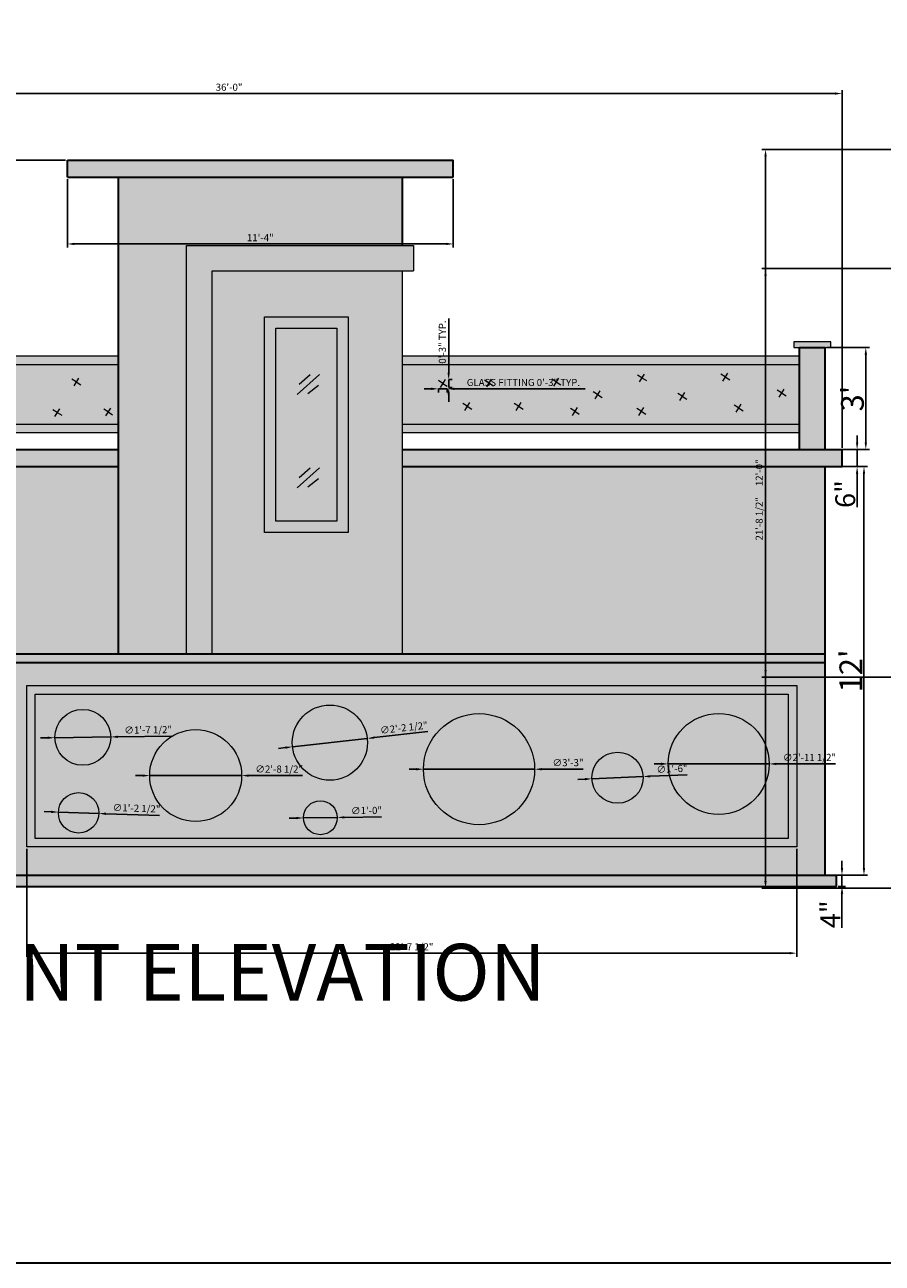
# Model space of a CAD drawing. Units: inches. Extents: x 2163 to 7246, y 928 to 2098.
# Tile 2 of 15: x 2404 to 2706, y 928 to 1365. Entities that reach past the tile are written whole.
import ezdxf

# ---------------------------------------------------------------- set-up
doc = ezdxf.new("R2010")
doc.units = ezdxf.units.IN
for name, color, linetype, lineweight in [('A-ANNO-DIMS', 4, 'Continuous', 18), ('A-ANNO-TITL', 4, 'Continuous', 30), ('A-ANNO-TTLB', 7, 'Continuous', 30), ('A-ELEV', 7, 'Continuous', 30), ('A-ELEV-DETL', 7, 'Continuous', 18), ('A-GLAZ', 30, 'Continuous', 20)]:
    doc.layers.add(name, color=color, linetype=linetype, lineweight=lineweight)
for name, color, linetype, lineweight, true_color in [('A-ELEV-PATT', 254, 'Continuous', 9, 0xd7ebd2), ('A-ELEV-TRIM-PATT', 11, 'Continuous', 9, 0xf27172), ('A-GLAZ-PATT', 141, 'Continuous', 9, 0xadddf7)]:
    doc.layers.add(name, color=color, linetype=linetype, lineweight=lineweight, true_color=true_color)
doc.styles.get("Standard").update_dxf_attribs({"font": 'arial.ttf'})
doc.dimstyles.new('ISO-25', dxfattribs={"dimtxt": 2.5, "dimasz": 2.5, "dimexe": 1.25, "dimexo": 0.625, "dimtad": 1, "dimdec": 0, "dimlunit": 3, "dimtxsty": 'Standard', "dimcen": 2.5, "dimadec": 0, "dimazin": 0, "dimtfac": 1, "dimtdec": 0, "dimtmove": 0, "dimatfit": 3, "dimfxl": 1, "dimarcsym": 0})

# ---------------------------------------------------------------- blocks, each defined once
blk = doc.blocks.new('*D21')
at = {"layer": 'A-ANNO-DIMS', "color": 0, "lineweight": -2, "transparency": 16777216}
for p, q in [((2691.82, 1067.77), (2691.82, 1070.27)), ((2690.47, 1065.27), (2693.07, 1065.27)), ((2691.82, 1065.27), (2691.82, 1061.27)), ((2690.47, 1061.27), (2693.07, 1061.27)), ((2691.82, 1058.77), (2691.82, 1046.7))]:
    blk.add_line(p, q, dxfattribs=at)
at = {"layer": 'A-ANNO-DIMS', "color": 0, "transparency": 16777216}
for points in [[(2691.4, 1067.77), (2692.24, 1067.77), (2691.82, 1065.27)], [(2691.4, 1058.77), (2692.24, 1058.77), (2691.82, 1061.27)]]:
    blk.add_solid(points, dxfattribs=at)
at = {"layer": 'Defpoints', "color": 0, "transparency": 16777216}
for p in [(2689.84, 1065.27), (2689.84, 1061.27), (2691.82, 1061.27)]:
    blk.add_point(p, dxfattribs=at)
at = {"layer": 'A-ANNO-DIMS', "color": 0, "transparency": 16777216, "insert": (2687.7, 1051.48), "char_height": 2.5, "attachment_point": 5, "rotation": 90}
blk.add_mtext('{\\H2.8x;4"}', dxfattribs=at)
blk = doc.blocks.new('*D22')
at = {"layer": 'A-ANNO-DIMS', "color": 0, "lineweight": -2, "transparency": 16777216}
for p, q in [((2686.47, 1209.27), (2700.82, 1209.27)), ((2699.57, 1206.77), (2699.57, 1067.77)), ((2686.47, 1065.27), (2700.82, 1065.27))]:
    blk.add_line(p, q, dxfattribs=at)
at = {"layer": 'A-ANNO-DIMS', "color": 0, "transparency": 16777216}
for points in [[(2699.15, 1206.77), (2699.98, 1206.77), (2699.57, 1209.27)], [(2699.15, 1067.77), (2699.98, 1067.77), (2699.57, 1065.27)]]:
    blk.add_solid(points, dxfattribs=at)
at = {"layer": 'Defpoints', "color": 0, "transparency": 16777216}
for p in [(2685.84, 1209.27), (2685.84, 1065.27), (2699.57, 1065.27)]:
    blk.add_point(p, dxfattribs=at)
at = {"layer": 'A-ANNO-DIMS', "color": 0, "transparency": 16777216, "insert": (2694.93, 1137.27), "char_height": 2.5, "attachment_point": 5, "rotation": 90}
blk.add_mtext("{\\H3.2x;12'}", dxfattribs=at)
blk = doc.blocks.new('*D23')
at = {"layer": 'A-ANNO-DIMS', "color": 0, "lineweight": -2, "transparency": 16777216}
for p, q in [((2697.15, 1217.77), (2697.15, 1220.27)), ((2692.47, 1215.27), (2698.4, 1215.27)), ((2697.15, 1215.27), (2697.15, 1209.27)), ((2692.47, 1209.27), (2698.4, 1209.27)), ((2697.15, 1206.77), (2697.15, 1194.94))]:
    blk.add_line(p, q, dxfattribs=at)
at = {"layer": 'A-ANNO-DIMS', "color": 0, "transparency": 16777216}
for points in [[(2696.74, 1217.77), (2697.57, 1217.77), (2697.15, 1215.27)], [(2696.74, 1206.77), (2697.57, 1206.77), (2697.15, 1209.27)]]:
    blk.add_solid(points, dxfattribs=at)
at = {"layer": 'Defpoints', "color": 0, "transparency": 16777216}
for p in [(2691.84, 1215.27), (2691.84, 1209.27), (2697.15, 1209.27)]:
    blk.add_point(p, dxfattribs=at)
at = {"layer": 'A-ANNO-DIMS', "color": 0, "transparency": 16777216, "insert": (2692.96, 1199.61), "char_height": 2.5, "attachment_point": 5, "rotation": 90}
blk.add_mtext('{\\H2.8x;6"}', dxfattribs=at)
blk = doc.blocks.new('*D24')
at = {"layer": 'A-ANNO-DIMS', "color": 0, "lineweight": -2, "transparency": 16777216}
for p, q in [((2686.47, 1251.27), (2701.46, 1251.27)), ((2700.21, 1248.77), (2700.21, 1217.77)), ((2686.47, 1215.27), (2701.46, 1215.27))]:
    blk.add_line(p, q, dxfattribs=at)
at = {"layer": 'A-ANNO-DIMS', "color": 0, "transparency": 16777216}
for points in [[(2699.8, 1248.77), (2700.63, 1248.77), (2700.21, 1251.27)], [(2699.8, 1217.77), (2700.63, 1217.77), (2700.21, 1215.27)]]:
    blk.add_solid(points, dxfattribs=at)
at = {"layer": 'Defpoints', "color": 0, "transparency": 16777216}
for p in [(2685.84, 1251.27), (2685.84, 1215.27), (2700.21, 1215.27)]:
    blk.add_point(p, dxfattribs=at)
at = {"layer": 'A-ANNO-DIMS', "color": 0, "transparency": 16777216, "insert": (2695.5, 1233.27), "char_height": 2.5, "attachment_point": 5, "rotation": 90}
blk.add_mtext("{\\H3.2x;3'}", dxfattribs=at)
blk = doc.blocks.new('GLASS-PANEL-FITTING')
for p, q in [((1.52, 1.46), (0, 2.43)), ((2.35, 2.77), (0.6, 0)), ((1.52, 1.46), (3.15, 0.44))]:
    blk.add_line(p, q)
blk = doc.blocks.new('GLAZ-REFLECTION')
for p, q in [((0, 0), (7.81, 7.08)), ((0.72, 3.7), (4.52, 7.08)), ((3.8, 0.41), (7.5, 3.29))]:
    blk.add_line(p, q)
blk = doc.blocks.new('*D47')
at = {"layer": 'A-ANNO-DIMS', "color": 0, "lineweight": -2, "transparency": 16777216}
for p, q in [((2547.09, 1236.69), (2544.59, 1236.69)), ((2549.59, 1236.69), (2552.74, 1236.69)), ((2549.59, 1236.54), (2549.59, 1235.44)), ((2552.74, 1236.54), (2552.74, 1235.44)), ((2555.24, 1236.69), (2601.36, 1236.69))]:
    blk.add_line(p, q, dxfattribs=at)
at = {"layer": 'A-ANNO-DIMS', "color": 0, "transparency": 16777216}
for points in [[(2547.09, 1237.11), (2547.09, 1236.28), (2549.59, 1236.69)], [(2555.24, 1237.11), (2555.24, 1236.28), (2552.74, 1236.69)]]:
    blk.add_solid(points, dxfattribs=at)
at = {"layer": 'Defpoints', "color": 0, "transparency": 16777216}
for p in [(2549.59, 1237.17), (2552.74, 1237.17), (2552.74, 1236.69)]:
    blk.add_point(p, dxfattribs=at)
at = {"layer": 'A-ANNO-DIMS', "color": 0, "transparency": 16777216, "insert": (2579.55, 1238.61), "char_height": 2.5, "attachment_point": 5}
blk.add_mtext('GLASS FITTING 0\'-3" TYP.', dxfattribs=at)
blk = doc.blocks.new('*D48')
at = {"layer": 'A-ANNO-DIMS', "color": 0, "lineweight": -2, "transparency": 16777216}
for p, q in [((2553.22, 1242.44), (2553.22, 1261.43)), ((2553.22, 1237.17), (2553.22, 1239.94)), ((2553.37, 1239.94), (2554.47, 1239.94)), ((2553.37, 1237.17), (2554.47, 1237.17)), ((2553.22, 1234.67), (2553.22, 1232.17))]:
    blk.add_line(p, q, dxfattribs=at)
at = {"layer": 'A-ANNO-DIMS', "color": 0, "transparency": 16777216}
for points in [[(2552.8, 1242.44), (2553.63, 1242.44), (2553.22, 1239.94)], [(2552.8, 1234.67), (2553.63, 1234.67), (2553.22, 1237.17)]]:
    blk.add_solid(points, dxfattribs=at)
at = {"layer": 'Defpoints', "color": 0, "transparency": 16777216}
for p in [(2552.74, 1239.94), (2553.22, 1239.94), (2552.74, 1237.17)]:
    blk.add_point(p, dxfattribs=at)
at = {"layer": 'A-ANNO-DIMS', "color": 0, "transparency": 16777216, "insert": (2551.31, 1253.18), "char_height": 2.5, "attachment_point": 5, "rotation": 90}
blk.add_mtext('0\'-3" TYP.', dxfattribs=at)
blk = doc.blocks.new('*D93')
at = {"layer": 'A-ANNO-DIMS', "color": 0, "lineweight": -2, "transparency": 16777216}
for p, q in [((2259.84, 1215.9), (2259.84, 1342.02)), ((2262.34, 1340.77), (2689.34, 1340.77)), ((2691.84, 1215.9), (2691.84, 1342.02))]:
    blk.add_line(p, q, dxfattribs=at)
at = {"layer": 'A-ANNO-DIMS', "color": 0, "transparency": 16777216}
for points in [[(2262.34, 1341.19), (2262.34, 1340.36), (2259.84, 1340.77)], [(2689.34, 1341.19), (2689.34, 1340.36), (2691.84, 1340.77)]]:
    blk.add_solid(points, dxfattribs=at)
at = {"layer": 'Defpoints', "color": 0, "transparency": 16777216}
for p in [(2691.84, 1340.77), (2259.84, 1215.27), (2691.84, 1215.27)]:
    blk.add_point(p, dxfattribs=at)
at = {"layer": 'A-ANNO-DIMS', "color": 0, "transparency": 16777216, "insert": (2475.84, 1342.68), "char_height": 2.5, "attachment_point": 5}
blk.add_mtext('36\'-0"', dxfattribs=at)
blk = doc.blocks.new('*D94')
at = {"layer": 'A-ANNO-DIMS', "color": 0, "lineweight": -2, "transparency": 16777216}
for p, q in [((2418.22, 1317.27), (2235.09, 1317.27)), ((2236.34, 1314.77), (2236.34, 1063.77)), ((2261.22, 1061.27), (2235.09, 1061.27))]:
    blk.add_line(p, q, dxfattribs=at)
at = {"layer": 'A-ANNO-DIMS', "color": 0, "transparency": 16777216}
for points in [[(2235.93, 1314.77), (2236.76, 1314.77), (2236.34, 1317.27)], [(2235.93, 1063.77), (2236.76, 1063.77), (2236.34, 1061.27)]]:
    blk.add_solid(points, dxfattribs=at)
at = {"layer": 'Defpoints', "color": 0, "transparency": 16777216}
for p in [(2418.84, 1317.27), (2236.34, 1061.27), (2261.84, 1061.27)]:
    blk.add_point(p, dxfattribs=at)
at = {"layer": 'A-ANNO-DIMS', "color": 0, "transparency": 16777216, "insert": (2234.46, 1189.27), "char_height": 2.5, "attachment_point": 5, "rotation": 90}
blk.add_mtext('21\'-4"', dxfattribs=at)
blk = doc.blocks.new('*D95')
at = {"layer": 'A-ANNO-DIMS', "color": 0, "lineweight": -2, "transparency": 16777216}
for p, q in [((2418.84, 1310.65), (2418.84, 1286.52)), ((2554.84, 1310.65), (2554.84, 1286.52)), ((2552.34, 1287.77), (2421.34, 1287.77))]:
    blk.add_line(p, q, dxfattribs=at)
at = {"layer": 'A-ANNO-DIMS', "color": 0, "transparency": 16777216}
for points in [[(2421.34, 1288.19), (2421.34, 1287.36), (2418.84, 1287.77)], [(2552.34, 1288.19), (2552.34, 1287.36), (2554.84, 1287.77)]]:
    blk.add_solid(points, dxfattribs=at)
at = {"layer": 'Defpoints', "color": 0, "transparency": 16777216}
for p in [(2418.84, 1311.27), (2554.84, 1311.27), (2418.84, 1287.77)]:
    blk.add_point(p, dxfattribs=at)
at = {"layer": 'A-ANNO-DIMS', "color": 0, "transparency": 16777216, "insert": (2486.84, 1289.65), "char_height": 2.5, "attachment_point": 5}
blk.add_mtext('11\'-4"', dxfattribs=at)
blk = doc.blocks.new('*D99')
at = {"layer": 'A-ANNO-DIMS', "color": 0, "lineweight": -2, "transparency": 16777216}
for p, q in [((2404.51, 1074.6), (2404.51, 1036.52)), ((2675.86, 1074.6), (2675.86, 1036.52)), ((2407.01, 1037.77), (2673.36, 1037.77))]:
    blk.add_line(p, q, dxfattribs=at)
at = {"layer": 'A-ANNO-DIMS', "color": 0, "transparency": 16777216}
for points in [[(2407.01, 1038.19), (2407.01, 1037.36), (2404.51, 1037.77)], [(2673.36, 1038.19), (2673.36, 1037.36), (2675.86, 1037.77)]]:
    blk.add_solid(points, dxfattribs=at)
at = {"layer": 'Defpoints', "color": 0, "transparency": 16777216}
for p in [(2404.51, 1075.23), (2675.86, 1075.23), (2675.86, 1037.77)]:
    blk.add_point(p, dxfattribs=at)
at = {"layer": 'A-ANNO-DIMS', "color": 0, "transparency": 16777216, "insert": (2540.19, 1039.69), "char_height": 2.5, "attachment_point": 5}
blk.add_mtext('22\'-7 1/2"', dxfattribs=at)
blk = doc.blocks.new('*D101')
at = {"layer": 'A-ANNO-DIMS', "color": 0, "lineweight": -2, "transparency": 16777216}
for p, q in [((2773.92, 1321.11), (2663.63, 1321.11)), ((2664.88, 1318.61), (2664.88, 1063.18)), ((2749.92, 1060.68), (2663.63, 1060.68))]:
    blk.add_line(p, q, dxfattribs=at)
at = {"layer": 'A-ANNO-DIMS', "color": 0, "transparency": 16777216}
for points in [[(2664.46, 1318.61), (2665.3, 1318.61), (2664.88, 1321.11)], [(2664.46, 1063.18), (2665.3, 1063.18), (2664.88, 1060.68)]]:
    blk.add_solid(points, dxfattribs=at)
at = {"layer": 'Defpoints', "color": 0, "transparency": 16777216}
for p in [(2774.54, 1321.11), (2664.88, 1060.68), (2750.54, 1060.68)]:
    blk.add_point(p, dxfattribs=at)
at = {"layer": 'A-ANNO-DIMS', "color": 0, "transparency": 16777216, "insert": (2662.96, 1190.89), "char_height": 2.5, "attachment_point": 5, "rotation": 90}
blk.add_mtext('21\'-8 1/2"', dxfattribs=at)
blk = doc.blocks.new('*D107')
at = {"layer": 'A-ANNO-DIMS', "color": 0, "lineweight": -2, "transparency": 16777216}
for p, q in [((3256.92, 1279.11), (2663.63, 1279.11)), ((2664.88, 1137.61), (2664.88, 1276.61)), ((3256.92, 1135.11), (2663.63, 1135.11))]:
    blk.add_line(p, q, dxfattribs=at)
at = {"layer": 'A-ANNO-DIMS', "color": 0, "transparency": 16777216}
for points in [[(2664.46, 1276.61), (2665.3, 1276.61), (2664.88, 1279.11)], [(2664.46, 1137.61), (2665.3, 1137.61), (2664.88, 1135.11)]]:
    blk.add_solid(points, dxfattribs=at)
at = {"layer": 'Defpoints', "color": 0, "transparency": 16777216}
for p in [(2664.88, 1279.11), (3257.54, 1279.11), (3257.54, 1135.11)]:
    blk.add_point(p, dxfattribs=at)
at = {"layer": 'A-ANNO-DIMS', "color": 0, "transparency": 16777216, "insert": (2662.98, 1207.11), "char_height": 2.5, "attachment_point": 5, "rotation": 90}
blk.add_mtext('12\'-0"', dxfattribs=at)
blk = doc.blocks.new('*D121')
at = {"layer": 'A-ANNO-DIMS', "color": 0, "lineweight": -2, "transparency": 16777216}
for p, q in [((2411.93, 1113.69), (2409.43, 1113.66)), ((2414.43, 1113.73), (2434.12, 1114)), ((2455.56, 1114.3), (2436.62, 1114.04))]:
    blk.add_line(p, q, dxfattribs=at)
at = {"layer": 'A-ANNO-DIMS', "color": 0, "transparency": 16777216}
for points in [[(2411.92, 1114.11), (2411.93, 1113.28), (2414.43, 1113.73)], [(2436.62, 1114.45), (2436.63, 1113.62), (2434.12, 1114)]]:
    blk.add_solid(points, dxfattribs=at)
at = {"layer": 'Defpoints', "color": 0, "transparency": 16777216}
for p in [(2414.43, 1113.73), (2434.12, 1114)]:
    blk.add_point(p, dxfattribs=at)
at = {"layer": 'A-ANNO-DIMS', "color": 0, "transparency": 16777216, "insert": (2447.32, 1116.16), "char_height": 2.5, "attachment_point": 5, "rotation": 0.7959}
blk.add_mtext('∅1\'-7 1/2"', dxfattribs=at)
blk = doc.blocks.new('*D122')
at = {"layer": 'A-ANNO-DIMS', "color": 0, "lineweight": -2, "transparency": 16777216}
for p, q in [((2413.19, 1087.57), (2410.69, 1087.66)), ((2415.68, 1087.49), (2429.93, 1087)), ((2451.36, 1086.27), (2432.43, 1086.92))]:
    blk.add_line(p, q, dxfattribs=at)
at = {"layer": 'A-ANNO-DIMS', "color": 0, "transparency": 16777216}
for points in [[(2413.2, 1087.99), (2413.17, 1087.15), (2415.68, 1087.49)], [(2432.45, 1087.33), (2432.42, 1086.5), (2429.93, 1087)]]:
    blk.add_solid(points, dxfattribs=at)
at = {"layer": 'Defpoints', "color": 0, "transparency": 16777216}
for p in [(2415.68, 1087.49), (2429.93, 1087)]:
    blk.add_point(p, dxfattribs=at)
at = {"layer": 'A-ANNO-DIMS', "color": 0, "transparency": 16777216, "insert": (2443.21, 1088.52), "char_height": 2.5, "attachment_point": 5, "rotation": 358.055}
blk.add_mtext('∅1\'-2 1/2"', dxfattribs=at)
blk = doc.blocks.new('*D123')
at = {"layer": 'A-ANNO-DIMS', "color": 0, "lineweight": -2, "transparency": 16777216}
for p, q in [((2445.37, 1100.37), (2442.87, 1100.37)), ((2447.87, 1100.37), (2480.27, 1100.37)), ((2501.71, 1100.37), (2482.77, 1100.37))]:
    blk.add_line(p, q, dxfattribs=at)
at = {"layer": 'A-ANNO-DIMS', "color": 0, "transparency": 16777216}
for points in [[(2445.37, 1100.78), (2445.37, 1099.95), (2447.87, 1100.37)], [(2482.77, 1100.78), (2482.77, 1099.95), (2480.27, 1100.37)]]:
    blk.add_solid(points, dxfattribs=at)
at = {"layer": 'Defpoints', "color": 0, "transparency": 16777216}
for p in [(2447.87, 1100.37), (2480.27, 1100.37)]:
    blk.add_point(p, dxfattribs=at)
at = {"layer": 'A-ANNO-DIMS', "color": 0, "transparency": 16777216, "insert": (2493.49, 1102.34), "char_height": 2.5, "attachment_point": 5, "rotation": 359.9996}
blk.add_mtext('∅2\'-8 1/2"', dxfattribs=at)
blk = doc.blocks.new('*D124')
at = {"layer": 'A-ANNO-DIMS', "color": 0, "lineweight": -2, "transparency": 16777216}
for p, q in [((2498.19, 1110.51), (2524.54, 1113.47)), ((2545.85, 1115.86), (2527.02, 1113.75)), ((2495.7, 1110.23), (2493.22, 1109.95))]:
    blk.add_line(p, q, dxfattribs=at)
at = {"layer": 'A-ANNO-DIMS', "color": 0, "transparency": 16777216}
for points in [[(2526.98, 1114.16), (2527.07, 1113.34), (2524.54, 1113.47)], [(2495.66, 1110.64), (2495.75, 1109.82), (2498.19, 1110.51)]]:
    blk.add_solid(points, dxfattribs=at)
at = {"layer": 'Defpoints', "color": 0, "transparency": 16777216}
for p in [(2524.54, 1113.47), (2498.19, 1110.51)]:
    blk.add_point(p, dxfattribs=at)
at = {"layer": 'A-ANNO-DIMS', "color": 0, "transparency": 16777216, "insert": (2537.46, 1116.91), "char_height": 2.5, "attachment_point": 5, "rotation": 6.4111}
blk.add_mtext('∅2\'-2 1/2"', dxfattribs=at)
blk = doc.blocks.new('*D125')
at = {"layer": 'A-ANNO-DIMS', "color": 0, "lineweight": -2, "transparency": 16777216}
for p, q in [((2499.52, 1085.4), (2497.02, 1085.37)), ((2502.02, 1085.44), (2513.98, 1085.61)), ((2529.59, 1085.83), (2516.48, 1085.64))]:
    blk.add_line(p, q, dxfattribs=at)
at = {"layer": 'A-ANNO-DIMS', "color": 0, "transparency": 16777216}
for points in [[(2499.51, 1085.82), (2499.52, 1084.99), (2502.02, 1085.44)], [(2516.47, 1086.06), (2516.49, 1085.23), (2513.98, 1085.61)]]:
    blk.add_solid(points, dxfattribs=at)
at = {"layer": 'Defpoints', "color": 0, "transparency": 16777216}
for p in [(2502.02, 1085.44), (2513.98, 1085.61)]:
    blk.add_point(p, dxfattribs=at)
at = {"layer": 'A-ANNO-DIMS', "color": 0, "transparency": 16777216, "insert": (2524.26, 1087.72), "char_height": 2.5, "attachment_point": 5, "rotation": 0.8105}
blk.add_mtext('∅1\'-0"', dxfattribs=at)
blk = doc.blocks.new('*D126')
at = {"layer": 'A-ANNO-DIMS', "color": 0, "lineweight": -2, "transparency": 16777216}
for p, q in [((2541.82, 1102.62), (2539.32, 1102.62)), ((2544.32, 1102.62), (2583.51, 1102.62)), ((2600.57, 1102.62), (2586.01, 1102.62))]:
    blk.add_line(p, q, dxfattribs=at)
at = {"layer": 'A-ANNO-DIMS', "color": 0, "transparency": 16777216}
for points in [[(2541.82, 1103.03), (2541.82, 1102.2), (2544.32, 1102.62)], [(2586.01, 1103.03), (2586.01, 1102.2), (2583.51, 1102.62)]]:
    blk.add_solid(points, dxfattribs=at)
at = {"layer": 'Defpoints', "color": 0, "transparency": 16777216}
for p in [(2544.32, 1102.62), (2583.51, 1102.62)]:
    blk.add_point(p, dxfattribs=at)
at = {"layer": 'A-ANNO-DIMS', "color": 0, "transparency": 16777216, "insert": (2595.27, 1104.59), "char_height": 2.5, "attachment_point": 5, "rotation": 0.0007}
blk.add_mtext('∅3\'-3"', dxfattribs=at)
blk = doc.blocks.new('*D127')
at = {"layer": 'A-ANNO-DIMS', "color": 0, "lineweight": -2, "transparency": 16777216}
for p, q in [((2637.31, 1100.69), (2624.21, 1100.12)), ((2601.22, 1099.12), (2598.72, 1099.01)), ((2603.72, 1099.23), (2621.71, 1100.01))]:
    blk.add_line(p, q, dxfattribs=at)
at = {"layer": 'A-ANNO-DIMS', "color": 0, "transparency": 16777216}
for points in [[(2624.19, 1100.53), (2624.23, 1099.7), (2621.71, 1100.01)], [(2601.2, 1099.53), (2601.24, 1098.7), (2603.72, 1099.23)]]:
    blk.add_solid(points, dxfattribs=at)
at = {"layer": 'Defpoints', "color": 0, "transparency": 16777216}
for p in [(2603.72, 1099.23), (2621.71, 1100.01)]:
    blk.add_point(p, dxfattribs=at)
at = {"layer": 'A-ANNO-DIMS', "color": 0, "transparency": 16777216, "insert": (2631.93, 1102.43), "char_height": 2.5, "attachment_point": 5, "rotation": 2.495}
blk.add_mtext('∅1\'-6"', dxfattribs=at)
blk = doc.blocks.new('*D128')
at = {"layer": 'A-ANNO-DIMS', "color": 0, "lineweight": -2, "transparency": 16777216}
for p, q in [((2628.09, 1104.49), (2625.59, 1104.49)), ((2630.59, 1104.49), (2666.17, 1104.49)), ((2689.55, 1104.49), (2668.67, 1104.49))]:
    blk.add_line(p, q, dxfattribs=at)
at = {"layer": 'A-ANNO-DIMS', "color": 0, "transparency": 16777216}
for points in [[(2628.09, 1104.91), (2628.09, 1104.08), (2630.59, 1104.49)], [(2668.67, 1104.91), (2668.67, 1104.07), (2666.17, 1104.49)]]:
    blk.add_solid(points, dxfattribs=at)
at = {"layer": 'Defpoints', "color": 0, "transparency": 16777216}
for p in [(2630.59, 1104.49), (2666.17, 1104.49)]:
    blk.add_point(p, dxfattribs=at)
at = {"layer": 'A-ANNO-DIMS', "color": 0, "transparency": 16777216, "insert": (2680.36, 1106.46), "char_height": 2.5, "attachment_point": 5, "rotation": 359.9986}
blk.add_mtext('∅2\'-11 1/2"', dxfattribs=at)

msp = doc.modelspace()

# ---------------------------------------------------------------- hatches: boundary and pattern name
at = {"layer": 'A-ELEV-PATT'}
h = msp.add_hatch(color=256, dxfattribs=at)
h.dxf.hatch_style = 1
h.paths.add_polyline_path([(2460.84, 1287.27), (2536.84, 1287.27), (2536.84, 1311.27), (2436.84, 1311.27), (2436.84, 1215.27), (2436.84, 1143.27), (2460.84, 1143.27), (2460.84, 1215.27)])
h = msp.add_hatch(color=256, dxfattribs=at)
h.dxf.hatch_style = 1
h.paths.add_polyline_path([(2536.84, 1278.27), (2469.84, 1278.27), (2469.84, 1215.27), (2469.84, 1143.27), (2536.84, 1143.27)])
h.paths.add_polyline_path([(2488.32, 1186.07), (2488.32, 1262.03), (2517.83, 1262.03), (2517.83, 1186.07)], flags=16)
h.paths.add_polyline_path([(2513.83, 1190.07), (2492.32, 1190.07), (2492.32, 1258.03), (2513.83, 1258.03)], flags=0)
h = msp.add_hatch(color=256, dxfattribs=at)
h.dxf.hatch_style = 1
h.paths.add_polyline_path([(2685.84, 1251.27), (2676.84, 1251.27), (2676.84, 1215.27), (2685.84, 1215.27)])
h = msp.add_hatch(color=256, dxfattribs=at)
h.dxf.hatch_style = 1
h.paths.add_polyline_path([(2436.84, 1209.27), (2265.84, 1209.27), (2265.84, 1143.27), (2319.84, 1143.27), (2319.84, 1140.27), (2313.84, 1140.27), (2313.84, 1125.27), (2355.84, 1125.27), (2355.84, 1137.27), (2385.84, 1137.27), (2385.84, 1140.27), (2379.84, 1140.27), (2379.84, 1143.27), (2436.84, 1143.27)])
h.paths.add_polyline_path([(2676.84, 1209.27), (2536.84, 1209.27), (2536.84, 1143.27), (2676.84, 1143.27)])
h = msp.add_hatch(color=256, dxfattribs=at)
h.dxf.hatch_style = 1
h.paths.add_polyline_path([(2685.84, 1209.27), (2536.84, 1209.27), (2536.84, 1143.27), (2676.84, 1143.27), (2685.84, 1143.27)])
h = msp.add_hatch(color=256, dxfattribs=at)
h.dxf.hatch_style = 1
h.paths.add_polyline_path([(2672.86, 1078.23), (2672.86, 1129.07), (2407.51, 1129.07), (2407.51, 1078.23)], flags=0)
h.paths.add_polyline_path([(2447.87, 1100.37, -1), (2480.27, 1100.37, -1)], flags=0)
h.paths.add_polyline_path([(2429.94, 1087.24, -1), (2415.68, 1087.24, -1)], flags=0)
h.paths.add_polyline_path([(2414.43, 1113.86, -1), (2434.12, 1113.86, -1)], flags=0)
h.paths.add_polyline_path([(2498.1, 1111.99, -1), (2524.62, 1111.99, -1)], flags=0)
h.paths.add_polyline_path([(2513.98, 1085.52, -1), (2502.02, 1085.52, -1)], flags=0)
h.paths.add_polyline_path([(2583.51, 1102.62, -1), (2544.32, 1102.62, -1)], flags=0)
h.paths.add_polyline_path([(2621.72, 1099.62, -1), (2603.71, 1099.62, -1)], flags=0)
h.paths.add_polyline_path([(2666.17, 1104.49, -1), (2630.59, 1104.49, -1)], flags=0)
h.paths.add_polyline_path([(2394.84, 1065.27), (2685.84, 1065.27), (2685.84, 1140.27), (2676.84, 1140.27), (2394.84, 1140.27)])
h.paths.add_polyline_path([(2404.51, 1132.07), (2675.86, 1132.07), (2675.86, 1075.23), (2404.51, 1075.23)], flags=16)
h.paths.add_polyline_path([(2407.51, 1129.07), (2672.86, 1129.07), (2672.86, 1078.23), (2407.51, 1078.23)], flags=0)
h = msp.add_hatch(color=256, dxfattribs=at)
h.dxf.hatch_style = 1
h.paths.add_polyline_path([(2672.86, 1078.23), (2672.86, 1129.07), (2407.51, 1129.07), (2407.51, 1078.23)])
h.paths.add_polyline_path([(2498.1, 1111.99, -1), (2524.62, 1111.99, -1)], flags=16)
h.paths.add_polyline_path([(2447.87, 1100.37, -1), (2480.27, 1100.37, -1)], flags=16)
h.paths.add_polyline_path([(2513.98, 1085.52, -1), (2502.02, 1085.52, -1)], flags=16)
h.paths.add_polyline_path([(2583.51, 1102.62, -1), (2544.32, 1102.62, -1)], flags=16)
h.paths.add_polyline_path([(2414.43, 1113.86, -1), (2434.12, 1113.86, -1)], flags=16)
h.paths.add_polyline_path([(2429.94, 1087.24, -1), (2415.68, 1087.24, -1)], flags=16)
h.paths.add_polyline_path([(2621.72, 1099.62, -1), (2603.71, 1099.62, -1)], flags=16)
h.paths.add_polyline_path([(2666.17, 1104.49, -1), (2630.59, 1104.49, -1)], flags=16)
at = {"layer": 'A-ELEV-TRIM-PATT'}
h = msp.add_hatch(color=256, dxfattribs=at)
h.dxf.hatch_style = 1
h.paths.add_polyline_path([(2418.84, 1317.27), (2418.84, 1311.27), (2554.84, 1311.27), (2554.84, 1317.27)])
h = msp.add_hatch(color=256, dxfattribs=at)
h.dxf.hatch_style = 1
h.paths.add_polyline_path([(2469.84, 1215.27), (2469.84, 1278.27), (2540.84, 1278.27), (2540.84, 1287.27), (2460.84, 1287.27), (2460.84, 1215.27), (2460.84, 1143.27), (2469.84, 1143.27)])
h = msp.add_hatch(color=256, dxfattribs=at)
h.dxf.hatch_style = 1
h.paths.add_polyline_path([(2488.32, 1186.07), (2517.83, 1186.07), (2517.83, 1262.03), (2488.32, 1262.03)])
h.paths.add_polyline_path([(2492.32, 1258.03), (2513.83, 1258.03), (2513.83, 1190.07), (2492.32, 1190.07)], flags=16)
h = msp.add_hatch(color=256, dxfattribs=at)
h.dxf.hatch_style = 1
h.paths.add_polyline_path([(2276.84, 1253.27), (2263.84, 1253.27), (2263.84, 1251.27), (2265.84, 1251.27), (2274.84, 1251.27), (2276.84, 1251.27)])
h.paths.add_polyline_path([(2687.84, 1253.27), (2676.84, 1253.27), (2674.84, 1253.27), (2674.84, 1251.27), (2676.84, 1251.27), (2685.84, 1251.27), (2687.84, 1251.27)])
h = msp.add_hatch(color=256, dxfattribs=at)
h.dxf.hatch_style = 1
h.paths.add_polyline_path([(2436.84, 1248.27), (2274.84, 1248.27), (2274.84, 1245.27), (2436.84, 1245.27)])
h.paths.add_polyline_path([(2436.84, 1224.27), (2274.84, 1224.27), (2274.84, 1221.27), (2436.84, 1221.27)])
h.paths.add_polyline_path([(2676.84, 1248.27), (2536.84, 1248.27), (2536.84, 1245.27), (2676.84, 1245.27)])
h.paths.add_polyline_path([(2676.84, 1224.27), (2536.84, 1224.27), (2536.84, 1221.27), (2676.84, 1221.27)])
h = msp.add_hatch(color=256, dxfattribs=at)
h.dxf.hatch_style = 1
h.paths.add_polyline_path([(2536.84, 1215.27), (2536.84, 1209.27), (2691.84, 1209.27), (2691.84, 1215.27)])
h.paths.add_polyline_path([(2259.84, 1215.27), (2259.84, 1209.27), (2436.84, 1209.27), (2436.84, 1215.27)])
h = msp.add_hatch(color=256, dxfattribs=at)
h.dxf.hatch_style = 1
h.paths.add_polyline_path([(2319.84, 1143.27), (2265.84, 1143.27), (2265.84, 1140.27), (2319.84, 1140.27)])
h.paths.add_polyline_path([(2676.84, 1143.27), (2379.84, 1143.27), (2379.84, 1140.27), (2676.84, 1140.27)])
h = msp.add_hatch(color=256, dxfattribs=at)
h.dxf.hatch_style = 1
h.paths.add_polyline_path([(2685.84, 1140.27), (2685.84, 1143.27), (2676.84, 1143.27), (2379.84, 1143.27), (2379.84, 1140.27), (2676.84, 1140.27)])
h = msp.add_hatch(color=256, dxfattribs=at)
h.dxf.hatch_style = 1
h.paths.add_polyline_path([(2404.51, 1075.23), (2675.86, 1075.23), (2675.86, 1132.07), (2404.51, 1132.07)])
h.paths.add_polyline_path([(2407.51, 1129.07), (2672.86, 1129.07), (2672.86, 1078.23), (2407.51, 1078.23)], flags=16)
h.paths.add_polyline_path([(2414.43, 1113.86, -1), (2434.12, 1113.86, -1)], flags=0)
h.paths.add_polyline_path([(2429.94, 1087.24, -1), (2415.68, 1087.24, -1)], flags=0)
h.paths.add_polyline_path([(2480.27, 1100.37, -1), (2447.87, 1100.37, -1)], flags=0)
h.paths.add_polyline_path([(2524.62, 1111.99, -1), (2498.1, 1111.99, -1)], flags=0)
h.paths.add_polyline_path([(2513.98, 1085.52, -1), (2502.02, 1085.52, -1)], flags=0)
h.paths.add_polyline_path([(2583.51, 1102.62, -1), (2544.32, 1102.62, -1)], flags=0)
h.paths.add_polyline_path([(2621.72, 1099.62, -1), (2603.71, 1099.62, -1)], flags=0)
h.paths.add_polyline_path([(2666.17, 1104.49, -1), (2630.59, 1104.49, -1)], flags=0)
h = msp.add_hatch(color=256, dxfattribs=at)
h.dxf.hatch_style = 1
h.paths.add_polyline_path([(2447.87, 1100.37, 1), (2480.27, 1100.37, 1)])
h.paths.add_polyline_path([(2524.62, 1111.99, 1), (2498.1, 1111.99, 1)])
h.paths.add_polyline_path([(2544.32, 1102.62, 1), (2583.51, 1102.62, 1)])
h.paths.add_polyline_path([(2603.71, 1099.62, 1), (2621.72, 1099.62, 1)])
h.paths.add_polyline_path([(2666.17, 1104.49, 1), (2630.59, 1104.49, 1)])
h.paths.add_polyline_path([(2415.68, 1087.24, 1), (2429.94, 1087.24, 1)])
h.paths.add_polyline_path([(2434.12, 1113.86, 1), (2414.43, 1113.86, 1)])
h = msp.add_hatch(color=256, dxfattribs=at)
h.dxf.hatch_style = 1
h.paths.add_polyline_path([(2502.02, 1085.52, 1), (2513.98, 1085.52, 1)])
h = msp.add_hatch(color=256, dxfattribs=at)
h.dxf.hatch_style = 1
h.paths.add_polyline_path([(2689.84, 1061.27), (2689.84, 1065.27), (2261.84, 1065.27), (2261.84, 1061.27)])
at = {"layer": 'A-GLAZ-PATT'}
h = msp.add_hatch(color=256, dxfattribs=at)
h.dxf.hatch_style = 1
h.paths.add_polyline_path([(2513.83, 1258.03), (2492.32, 1258.03), (2492.32, 1190.07), (2513.83, 1190.07)])
h = msp.add_hatch(color=256, dxfattribs=at)
h.dxf.hatch_style = 1
h.paths.add_polyline_path([(2436.84, 1224.27), (2436.84, 1245.27), (2274.84, 1245.27), (2274.84, 1224.27)])
h.paths.add_polyline_path([(2536.84, 1245.27), (2536.84, 1224.27), (2676.84, 1224.27), (2676.84, 1245.27)])

# ---------------------------------------------------------------- linework, layer by layer
at = {"layer": 'A-ANNO-TTLB'}
msp.add_lwpolyline([(2162.62, 2098.21), (3633.38, 2098.21), (3633.38, 928.48), (2162.62, 928.48)], close=True, dxfattribs=at)
at = {"layer": 'A-ELEV'}
for p, q in [((2418.84, 1317.27), (2554.84, 1317.27)), ((2418.84, 1311.27), (2418.84, 1317.27)), ((2554.84, 1311.27), (2554.84, 1317.27)), ((2418.84, 1311.27), (2554.84, 1311.27)), ((2436.84, 1215.27), (2436.84, 1311.27)), ((2536.84, 1311.27), (2536.84, 1287.27)), ((2676.84, 1251.27), (2685.84, 1251.27)), ((2676.84, 1215.27), (2676.84, 1251.27)), ((2685.84, 1215.27), (2685.84, 1251.27)), ((2259.84, 1215.27), (2436.84, 1215.27)), ((2436.84, 1143.27), (2436.84, 1215.27)), ((2536.84, 1215.27), (2691.84, 1215.27)), ((2691.84, 1209.27), (2691.84, 1215.27)), ((2259.84, 1209.27), (2436.84, 1209.27)), ((2536.84, 1209.27), (2691.84, 1209.27)), ((2685.84, 1065.27), (2685.84, 1209.27)), ((2379.84, 1143.27), (2676.84, 1143.27)), ((2379.84, 1140.27), (2676.84, 1140.27)), ((2676.84, 1143.27), (2685.84, 1143.27)), ((2676.84, 1140.27), (2685.84, 1140.27)), ((2261.84, 1065.27), (2689.84, 1065.27)), ((2689.84, 1061.27), (2689.84, 1065.27)), ((2261.84, 1061.27), (2689.84, 1061.27))]:
    msp.add_line(p, q, dxfattribs=at)
at = {"layer": 'A-ELEV-DETL'}
for p, q in [((2460.84, 1215.27), (2460.84, 1287.27)), ((2460.84, 1287.27), (2540.84, 1287.27)), ((2540.84, 1287.27), (2540.84, 1278.27)), ((2469.84, 1278.27), (2540.84, 1278.27)), ((2469.84, 1215.27), (2469.84, 1278.27)), ((2536.84, 1278.27), (2536.84, 1143.27)), ((2676.84, 1253.27), (2674.84, 1253.27)), ((2674.84, 1253.27), (2674.84, 1251.27)), ((2687.84, 1253.27), (2676.84, 1253.27)), ((2687.84, 1251.27), (2687.84, 1253.27)), ((2674.84, 1251.27), (2676.84, 1251.27)), ((2685.84, 1251.27), (2687.84, 1251.27)), ((2274.84, 1248.27), (2436.84, 1248.27)), ((2274.84, 1245.27), (2436.84, 1245.27)), ((2536.84, 1248.27), (2676.84, 1248.27)), ((2536.84, 1245.27), (2676.84, 1245.27)), ((2274.84, 1224.27), (2436.84, 1224.27)), ((2536.84, 1224.27), (2676.84, 1224.27)), ((2274.84, 1221.27), (2436.84, 1221.27)), ((2536.84, 1221.27), (2676.84, 1221.27)), ((2460.84, 1143.27), (2460.84, 1215.27)), ((2469.84, 1143.27), (2469.84, 1215.27))]:
    msp.add_line(p, q, dxfattribs=at)
for points in [[(2404.51, 1132.07), (2675.86, 1132.07), (2675.86, 1075.23), (2404.51, 1075.23)], [(2407.51, 1129.07), (2672.86, 1129.07), (2672.86, 1078.23), (2407.51, 1078.23)]]:
    msp.add_lwpolyline(points, close=True, dxfattribs=at)
for centre, radius in [((2424.28, 1113.86), 9.85), ((2511.36, 1111.99), 13.26), ((2563.92, 1102.62), 19.59), ((2648.38, 1104.49), 17.79), ((2464.07, 1100.37), 16.2), ((2612.72, 1099.62), 9.01), ((2422.81, 1087.24), 7.13), ((2508, 1085.52), 5.98)]:
    msp.add_circle(centre, radius, dxfattribs=at)
at = {"layer": 'A-GLAZ'}
for points in [[(2488.32, 1262.03), (2517.83, 1262.03), (2517.83, 1186.07), (2488.32, 1186.07)], [(2492.32, 1258.03), (2513.83, 1258.03), (2513.83, 1190.07), (2492.32, 1190.07)]]:
    msp.add_lwpolyline(points, close=True, dxfattribs=at)

# ---------------------------------------------------------------- block references
at = {"layer": 'A-ELEV-DETL'}
for p in [(2420.48, 1237.72), (2549.59, 1237.17), (2565.9, 1237.36), (2589.59, 1237.66), (2619.8, 1239.14), (2649.12, 1239.43), (2604.1, 1233.22), (2668.96, 1233.81), (2558.2, 1229.08), (2576.27, 1229.08), (2634.01, 1232.63), (2653.86, 1228.49), (2413.74, 1226.92), (2431.65, 1227.15), (2596.11, 1227.31), (2619.5, 1227.31)]:
    msp.add_blockref('GLASS-PANEL-FITTING', p, dxfattribs=at)
at = {"layer": 'A-GLAZ'}
for p in [(2499.84, 1234.64), (2499.84, 1201.79)]:
    msp.add_blockref('GLAZ-REFLECTION', p, dxfattribs=at)

# ---------------------------------------------------------------- texts
at = {"layer": 'A-ANNO-TITL', "insert": (2349.09, 1041.06), "char_height": 20, "attachment_point": 1}
msp.add_mtext_dynamic_manual_height_columns('FRONT ELEVATION', width=571.2399, gutter_width=12.5, heights=[0], dxfattribs=at)

# ---------------------------------------------------------------- dimensions: what is measured, and where the dimension line sits
at = {"layer": 'A-ANNO-DIMS'}
for base, p1, p2, picture, middle in [((2691.84, 1340.77), (2259.84, 1215.27), (2691.84, 1215.27), '*D93', (2475.84, 1342.68)), ((2675.8622, 1037.773), (2404.5127, 1075.2279), (2675.8622, 1075.2279), '*D99', (2540.1875, 1039.6907))]:
    dim = msp.add_linear_dim(base=base, p1=p1, p2=p2, dimstyle='ISO-25', override={"dimdec": 1, "dimlfac": 1, "dimrnd": 0, "dimzin": 1, "dimdsep": 46, "dimlunit": 4, "dimfrac": 2}, dxfattribs=at)
    dim.commit()
    dim.dimension.update_dxf_attribs({"geometry": picture, "text_midpoint": middle})
for base, p1, p2, angle, picture, middle in [((2664.88, 1060.68), (2774.54, 1321.11), (2750.54, 1060.68), 90, '*D101', (2662.96, 1190.89)), ((2236.34, 1061.27), (2418.84, 1317.27), (2261.84, 1061.27), 90, '*D94', (2234.46, 1189.27)), ((2418.84, 1287.77), (2554.84, 1311.27), (2418.84, 1311.27), 180, '*D95', (2486.84, 1289.65)), ((2664.88, 1279.11), (3257.54, 1135.11), (3257.54, 1279.11), 90, '*D107', (2662.98, 1207.11))]:
    dim = msp.add_linear_dim(base=base, p1=p1, p2=p2, angle=angle, dimstyle='ISO-25', override={"dimdec": 1, "dimlfac": 1, "dimrnd": 0, "dimzin": 1, "dimdsep": 46, "dimlunit": 4, "dimfrac": 2}, dxfattribs=at)
    dim.commit()
    dim.dimension.update_dxf_attribs({"geometry": picture, "text_midpoint": middle})
for base, p1, p2, text, override, picture, middle in [((2553.22, 1239.94), (2552.74, 1237.17), (2552.74, 1239.94), '<> TYP.', {"dimdec": 1, "dimlfac": 1, "dimrnd": 0, "dimzin": 1, "dimdsep": 46, "dimlunit": 4, "dimfrac": 2}, '*D48', (2551.31, 1253.18)), ((2700.21, 1215.27), (2685.84, 1251.27), (2685.84, 1215.27), '{\\H3.2x;<>}', {"dimclrd": 0, "dimclre": 0, "dimclrt": 0}, '*D24', (2695.5, 1233.27)), ((2697.15, 1209.27), (2691.84, 1215.27), (2691.84, 1209.27), '{\\H2.8x;<>}', {"dimclrd": 0, "dimclre": 0, "dimclrt": 0}, '*D23', (2692.96, 1199.61)), ((2699.57, 1065.27), (2685.84, 1209.27), (2685.84, 1065.27), '{\\H3.2x;<>}', {"dimclrd": 0, "dimclre": 0, "dimclrt": 0}, '*D22', (2694.93, 1137.27)), ((2691.82, 1061.27), (2689.84, 1065.27), (2689.84, 1061.27), '{\\H2.8x;<>}', {"dimclrd": 0, "dimclre": 0, "dimclrt": 0}, '*D21', (2687.7, 1051.48))]:
    dim = msp.add_linear_dim(base=base, p1=p1, p2=p2, angle=90, text=text, dimstyle='ISO-25', override=override, dxfattribs=at)
    dim.commit()
    dim.dimension.update_dxf_attribs({"geometry": picture, "text_midpoint": middle})
dim = msp.add_linear_dim(base=(2552.7435, 1236.6946), p1=(2549.5897, 1237.1677), p2=(2552.7435, 1237.1677), text='GLASS FITTING <> TYP.', dimstyle='ISO-25', override={"dimdec": 1, "dimlfac": 1, "dimrnd": 0, "dimzin": 1, "dimdsep": 46, "dimlunit": 4, "dimfrac": 2}, dxfattribs=at)
dim.commit()
dim.dimension.update_dxf_attribs({"geometry": '*D47', "text_midpoint": (2579.5512, 1238.6131)})
for p1, p2, picture, middle in [((2414.43, 1113.73), (2434.12, 1114), '*D121', (2447.34, 1114.19)), ((2498.19, 1110.51), (2524.54, 1113.47), '*D124', (2537.68, 1114.95)), ((2544.32, 1102.62), (2583.51, 1102.62), '*D126', (2595.27, 1102.62)), ((2415.68, 1087.49), (2429.93, 1087), '*D122', (2443.15, 1086.55))]:
    dim = msp.add_diameter_dim_2p(p1=p1, p2=p2, dimstyle='ISO-25', override={"dimdec": 1, "dimlfac": 1, "dimrnd": 0, "dimzin": 1, "dimdsep": 46, "dimlunit": 4, "dimfrac": 2}, dxfattribs=at)
    dim.commit()
    dim.dimension.update_dxf_attribs({"geometry": picture, "text_midpoint": middle, "dimtype": 163})
for p1, p2, picture, middle in [((2630.59, 1104.49), (2666.17, 1104.49), '*D128', (2680.36, 1104.49)), ((2447.87, 1100.37), (2480.27, 1100.37), '*D123', (2493.49, 1100.37)), ((2603.72, 1099.23), (2621.71, 1100.01), '*D127', (2632.01, 1100.46)), ((2502.02, 1085.44), (2513.98, 1085.61), '*D125', (2524.29, 1085.75))]:
    dim = msp.add_diameter_dim_2p(p1=p1, p2=p2, dimstyle='ISO-25', override={"dimdec": 1, "dimlfac": 1, "dimrnd": 0, "dimzin": 1, "dimdsep": 46, "dimlunit": 4, "dimfrac": 2}, dxfattribs=at)
    dim.commit()
    dim.dimension.update_dxf_attribs({"geometry": picture, "text_midpoint": middle})

doc.saveas('drawing.dxf')
